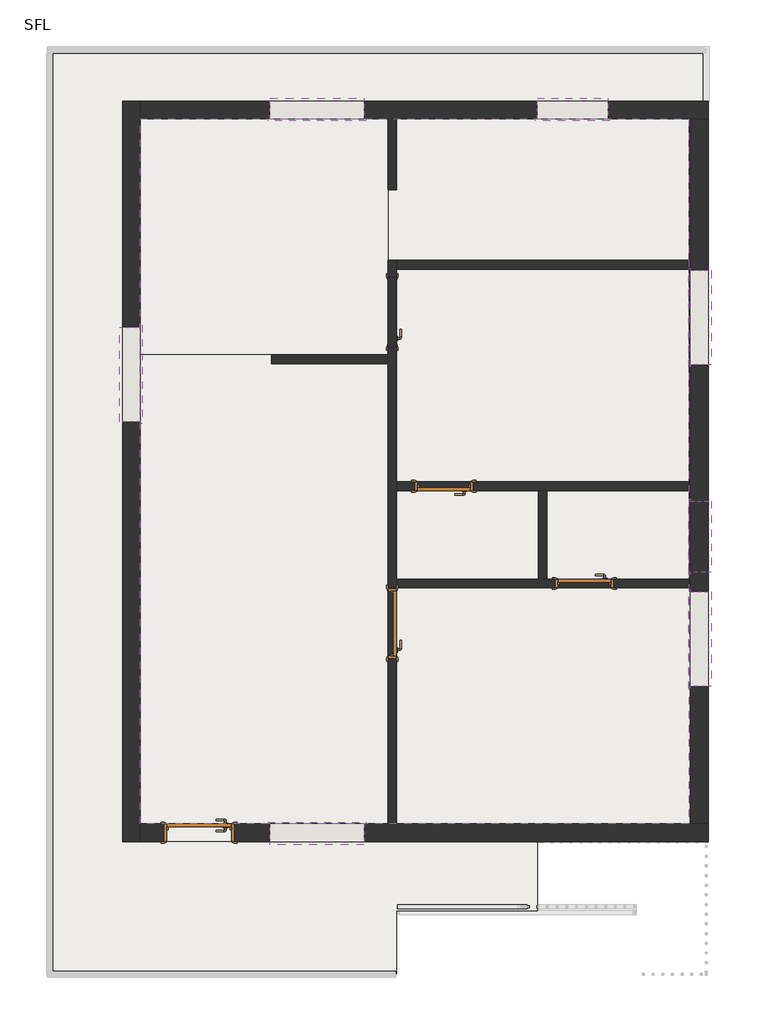
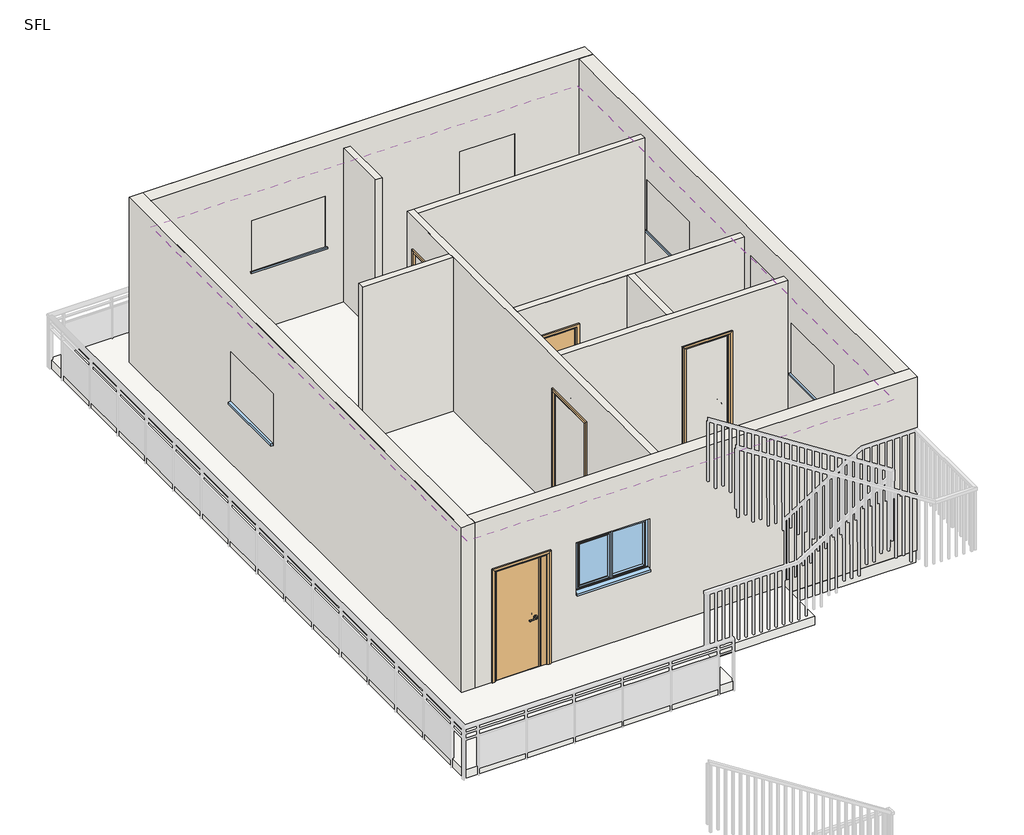
# One storey, part 1 of 4: 21 walls, 16 slabs, 7 windows, 5 doors, 1 covering.
"""IFC4 building model written with IfcOpenShell, lengths in millimetres."""

from ifc_helpers import new_model, si_unit, frame, origin, place, context, project, spatial, polyline, outline, extrude, faceted_brep, transform, mapped, element, save
from components import doors_intsgl_d1_d2de26da, doors_intsgl_d1_5aeab8eb, doors_intsgl_d2_21b53886, doors_intsgl_d2_1f5f3f16, windows_dbl_plain_w1_9e0d93ab, windows_dbl_plain_w2_c69f14ef, windows_sgl_plain_v_28d0678b

model = new_model("IFC4")

# Units and contexts
model_context = context("Model", 3, world=origin())
ifc_project = project(units=[si_unit("LENGTHUNIT", "METRE", prefix="MILLI")], contexts=[model_context])

# Site, building, storey
site = spatial("IfcSite", under=ifc_project)
building = spatial("IfcBuilding", under=site)
storey = spatial("IfcBuildingStorey", under=building, Name="SFL", Elevation=6583.68)

# Covering
placement = place(None, origin())
element("IfcCovering", 1, at=placement, inside=storey, context=model_context, shape_type="SweptSolid", body=[
    extrude(outline(polyline([(-6724.0132565, -885.5593981), (-6724.0132565, -9991.0521308), (-10495.9340108, -9991.0521308), (-13810.6009005, -9991.0521308), (-13810.6009005, -885.5593981), (-6724.0132565, -885.5593981)])), frame((0.0, 0.0, 9174.48), z_axis=(0.0, 0.0, 1.0), x_axis=(1.0, 0.0, 0.0)), (0.0, 0.0, 1.0), 57.0),
])

# Doors
doors_intsgl_d1_shape = doors_intsgl_d1_d2de26da(model_context)
element("IfcDoor", 2, ObjectType="Doors_IntSgl : D1", at=placement, inside=storey, context=model_context, shape_type="MappedRepresentation", body=[
    mapped(doors_intsgl_d1_shape, transform((-10553.0840108, -7400.866169, 6733.6416), x_axis=(0.0, 1.0, 0.0), y_axis=(-1.0, 0.0, 0.0), z_axis=(0.0, 0.0, 1.0))),
])
element("IfcDoor", 3, ObjectType="Doors_IntSgl : D1", at=placement, inside=storey, context=model_context, shape_type="MappedRepresentation", body=[
    mapped(doors_intsgl_d1_shape, transform((-10553.0840108, -3381.2262014, 6733.6416), x_axis=(0.0, 1.0, 0.0), y_axis=(-1.0, 0.0, 0.0), z_axis=(0.0, 0.0, 1.0))),
])
doors_intsgl_d1_2_shape = doors_intsgl_d1_5aeab8eb(model_context)
element("IfcDoor", 4, ObjectType="Doors_IntSgl : D1", at=placement, inside=storey, context=model_context, shape_type="MappedRepresentation", body=[
    mapped(doors_intsgl_d1_2_shape, transform((-13048.4335145, -10105.3521308, 6583.68), x_axis=(-1.0, 0.0, 0.0), y_axis=(0.0, -1.0, 0.0), z_axis=(0.0, 0.0, 1.0))),
])
doors_intsgl_d2_shape = doors_intsgl_d2_21b53886(model_context)
element("IfcDoor", 5, ObjectType="Doors_IntSgl : D2", at=placement, inside=storey, context=model_context, shape_type="MappedRepresentation", body=[
    mapped(doors_intsgl_d2_shape, transform((-9886.3340108, -5628.9784114, 6733.6416), x_axis=(-1.0, 0.0, 0.0), y_axis=(0.0, -1.0, 0.0), z_axis=(0.0, 0.0, 1.0))),
])
doors_intsgl_d2_2_shape = doors_intsgl_d2_1f5f3f16(model_context)
element("IfcDoor", 6, ObjectType="Doors_IntSgl : D2", at=placement, inside=storey, context=model_context, shape_type="MappedRepresentation", body=[
    mapped(doors_intsgl_d2_2_shape, transform((-8070.4366309, -6886.516169, 6733.6416), x_axis=(-1.0, 0.0, 0.0), y_axis=(0.0, -1.0, 0.0), z_axis=(0.0, 0.0, 1.0))),
])

# Slabs
element("IfcSlab", 7, ObjectType="BATHROOM FLOORING", at=placement, inside=storey, context=model_context, shape_type="SweptSolid", body=[
    extrude(outline(polyline([(-8667.3366309, -5686.1284114), (-8667.3366309, -6829.366169), (-10495.9340108, -6829.366169), (-10495.9340108, -5686.1284114), (-8667.3366309, -5686.1284114)])), frame((0.0, 0.0, 6583.68), z_axis=(0.0, 0.0, 1.0), x_axis=(1.0, 0.0, 0.0)), (0.0, 0.0, 1.0), 149.9616),
])
element("IfcSlab", 8, ObjectType="BATHROOM FLOORING", at=placement, inside=storey, context=model_context, shape_type="SweptSolid", body=[
    extrude(outline(polyline([(-6724.371003, -5686.0601635), (-6724.371003, -6829.366169), (-8553.0366309, -6829.366169), (-8553.0366309, -5686.0601635), (-6724.371003, -5686.0601635)])), frame((0.0, 0.0, 6583.68), z_axis=(0.0, 0.0, 1.0), x_axis=(1.0, 0.0, 0.0)), (0.0, 0.0, 1.0), 149.9616),
])
element("IfcSlab", 9, ObjectType="BATHROOM FLOORING", at=placement, inside=storey, context=model_context, shape_type="SweptSolid", body=[
    extrude(outline(polyline([(-8667.3366309, -5686.1284114), (-8667.3366309, -6829.366169), (-10495.9340108, -6829.366169), (-10495.9340108, -5686.1284114), (-8667.3366309, -5686.1284114)])), frame((0.0, 0.0, 6583.68), z_axis=(0.0, 0.0, 1.0), x_axis=(1.0, 0.0, 0.0)), (0.0, 0.0, 1.0), 149.9616),
])
element("IfcSlab", 10, ObjectType="BATHROOM FLOORING", at=placement, inside=storey, context=model_context, shape_type="SweptSolid", body=[
    extrude(outline(polyline([(-6724.371003, -5686.0601635), (-6724.371003, -6829.366169), (-8553.0366309, -6829.366169), (-8553.0366309, -5686.0601635), (-6724.371003, -5686.0601635)])), frame((0.0, 0.0, 6583.68), z_axis=(0.0, 0.0, 1.0), x_axis=(1.0, 0.0, 0.0)), (0.0, 0.0, 1.0), 149.9616),
])
element("IfcSlab", 11, ObjectType="BED ROOM FLOORING", at=placement, inside=storey, context=model_context, shape_type="SweptSolid", body=[
    extrude(outline(polyline([(-6724.371003, -2828.9136626), (-6724.371003, -5571.8284114), (-10495.9340108, -5571.8284114), (-10495.9340108, -2828.9136626), (-6724.371003, -2828.9136626)])), frame((0.0, 0.0, 6583.68), z_axis=(0.0, 0.0, 1.0), x_axis=(1.0, 0.0, 0.0)), (0.0, 0.0, 1.0), 149.9616),
])
element("IfcSlab", 12, ObjectType="BED ROOM FLOORING", at=placement, inside=storey, context=model_context, shape_type="SweptSolid", body=[
    extrude(outline(polyline([(-6698.6395131, -6943.5979211), (-6698.6395131, -9991.1886267), (-10495.9340108, -9991.1886267), (-10495.9340108, -6943.5979211), (-6698.6395131, -6943.5979211)])), frame((0.0, 0.0, 6583.68), z_axis=(0.0, 0.0, 1.0), x_axis=(1.0, 0.0, 0.0)), (0.0, 0.0, 1.0), 149.9616),
])
element("IfcSlab", 13, ObjectType="BED ROOM FLOORING", at=placement, inside=storey, context=model_context, shape_type="SweptSolid", body=[
    extrude(outline(polyline([(-6724.371003, -2828.9136626), (-6724.371003, -5571.8284114), (-10495.9340108, -5571.8284114), (-10495.9340108, -2828.9136626), (-6724.371003, -2828.9136626)])), frame((0.0, 0.0, 6583.68), z_axis=(0.0, 0.0, 1.0), x_axis=(1.0, 0.0, 0.0)), (0.0, 0.0, 1.0), 149.9616),
])
element("IfcSlab", 14, ObjectType="BED ROOM FLOORING", at=placement, inside=storey, context=model_context, shape_type="SweptSolid", body=[
    extrude(outline(polyline([(-6698.6395131, -6943.5979211), (-6698.6395131, -9991.1886267), (-10495.9340108, -9991.1886267), (-10495.9340108, -6943.5979211), (-6698.6395131, -6943.5979211)])), frame((0.0, 0.0, 6583.68), z_axis=(0.0, 0.0, 1.0), x_axis=(1.0, 0.0, 0.0)), (0.0, 0.0, 1.0), 149.9616),
])
element("IfcSlab", 15, ObjectType="DINING FLOORING", at=placement, inside=storey, context=model_context, shape_type="SweptSolid", body=[
    extrude(outline(polyline([(-10610.2340108, -885.9480347), (-10610.2340108, -3933.5387403), (-13810.6009005, -3933.5387403), (-13810.6009005, -885.9480347), (-10610.2340108, -885.9480347)])), frame((0.0, 0.0, 6583.68), z_axis=(0.0, 0.0, 1.0), x_axis=(1.0, 0.0, 0.0)), (0.0, 0.0, 1.0), 149.9616),
])
element("IfcSlab", 16, ObjectType="DINING FLOORING", at=placement, inside=storey, context=model_context, shape_type="SweptSolid", body=[
    extrude(outline(polyline([(-10610.2340108, -885.9480347), (-10610.2340108, -3933.5387403), (-13810.6009005, -3933.5387403), (-13810.6009005, -885.9480347), (-10610.2340108, -885.9480347)])), frame((0.0, 0.0, 6583.68), z_axis=(0.0, 0.0, 1.0), x_axis=(1.0, 0.0, 0.0)), (0.0, 0.0, 1.0), 149.9616),
])
element("IfcSlab", 17, ObjectType="HALL FLOORING", at=placement, inside=storey, context=model_context, shape_type="SweptSolid", body=[
    extrude(outline(polyline([(-10610.2340108, -3933.5387403), (-10610.2340108, -9991.0521308), (-13810.6009005, -9991.0521308), (-13810.6009005, -3933.5387403), (-10610.2340108, -3933.5387403)])), frame((0.0, 0.0, 6583.68), z_axis=(0.0, 0.0, 1.0), x_axis=(1.0, 0.0, 0.0)), (0.0, 0.0, 1.0), 149.9616),
])
element("IfcSlab", 18, ObjectType="HALL FLOORING", at=placement, inside=storey, context=model_context, shape_type="SweptSolid", body=[
    extrude(outline(polyline([(-10610.2340108, -3933.5387403), (-10610.2340108, -9991.0521308), (-13810.6009005, -9991.0521308), (-13810.6009005, -3933.5387403), (-10610.2340108, -3933.5387403)])), frame((0.0, 0.0, 6583.68), z_axis=(0.0, 0.0, 1.0), x_axis=(1.0, 0.0, 0.0)), (0.0, 0.0, 1.0), 149.9616),
])
element("IfcSlab", 19, ObjectType="KITCHEN FLOOR", at=placement, inside=storey, context=model_context, shape_type="SweptSolid", body=[
    extrude(outline(polyline([(-6724.371003, -885.9480347), (-6724.371003, -2714.6136626), (-10495.9340108, -2714.6136626), (-10610.2340108, -2714.6136626), (-10610.2340108, -1800.3480347), (-10495.9340108, -1800.3480347), (-10495.9340108, -885.9480347), (-6724.371003, -885.9480347)])), frame((0.0, 0.0, 6583.68), z_axis=(0.0, 0.0, 1.0), x_axis=(1.0, 0.0, 0.0)), (0.0, 0.0, 1.0), 149.9616),
])
element("IfcSlab", 20, ObjectType="KITCHEN FLOOR", at=placement, inside=storey, context=model_context, shape_type="SweptSolid", body=[
    extrude(outline(polyline([(-6724.371003, -885.9480347), (-6724.371003, -2714.6136626), (-10495.9340108, -2714.6136626), (-10610.2340108, -2714.6136626), (-10610.2340108, -1800.3480347), (-10495.9340108, -1800.3480347), (-10495.9340108, -885.9480347), (-6724.371003, -885.9480347)])), frame((0.0, 0.0, 6583.68), z_axis=(0.0, 0.0, 1.0), x_axis=(1.0, 0.0, 0.0)), (0.0, 0.0, 1.0), 149.9616),
])
element("IfcSlab", 21, ObjectType="OUTER FLOORING", at=placement, inside=storey, context=model_context, shape_type="SweptSolid", body=[
    extrude(outline(polyline([(-6495.4132565, 3.4571089), (-6495.4132565, -656.9593981), (-14039.0335145, -656.9593981), (-14039.0335145, -10219.6521308), (-8680.149573, -10219.6521308), (-8680.149573, -11109.5255223), (-10495.9340108, -11109.5255223), (-10495.9340108, -11928.1928911), (-14979.3420435, -11928.1928911), (-14979.3420435, 3.4571089), (-6495.4132565, 3.4571089)])), frame((0.0, 0.0, 6583.68), z_axis=(0.0, 0.0, 1.0), x_axis=(1.0, 0.0, 0.0)), (0.0, 0.0, 1.0), 149.9616),
])
element("IfcSlab", 22, ObjectType="RCC SLAB", at=placement, inside=storey, context=model_context, shape_type="SweptSolid", body=[
    extrude(outline(polyline([(-6495.4132565, -656.9593981), (-6495.4132565, -10219.6521308), (-14039.0335145, -10219.6521308), (-14039.0335145, -656.9593981), (-6495.4132565, -656.9593981)])), frame((0.0, 0.0, 6383.7312), z_axis=(0.0, 0.0, 1.0), x_axis=(1.0, 0.0, 0.0)), (0.0, 0.0, 1.0), 199.9488),
])

# Walls
element("IfcWall", 23, ObjectType="EXT WALL", at=placement, inside=storey, context=model_context, shape_type="Brep", body=[
    faceted_brep([(-14039.0335145, -656.9593981, 6583.68), (-14039.0335145, -10219.6521308, 6583.68), (-14039.0335145, -10219.6521308, 9631.68), (-14039.0335145, -656.9593981, 9631.68), (-14039.0335145, -4797.1593981, 8693.68), (-14039.0335145, -4797.1593981, 7783.68), (-14039.0335145, -3577.9593981, 7783.68), (-14039.0335145, -3577.9593981, 8693.68), (-13810.4335145, -656.9593981, 6583.68), (-13810.4335145, -656.9593981, 9631.68), (-13810.4335145, -885.5593981, 9631.68), (-13810.4335145, -9991.0521308, 9631.68), (-13810.4335145, -10219.6521308, 9631.68), (-13810.4335145, -10219.6521308, 6583.68), (-13810.4335145, -9991.0521308, 6583.68), (-13810.4335145, -885.5593981, 6583.68), (-13810.4335145, -4797.1593981, 8693.68), (-13810.4335145, -3577.9593981, 8693.68), (-13810.4335145, -3577.9593981, 7783.68), (-13810.4335145, -4797.1593981, 7783.68)], [[[0, 1, 2, 3], [4, 5, 6, 7]], [[8, 9, 10, 11, 12, 13, 14, 15], [16, 17, 18, 19]], [[1, 0, 8, 15, 14, 13]], [[3, 2, 12, 11, 10, 9]], [[2, 1, 13, 12]], [[0, 3, 9, 8]], [[5, 4, 16, 19]], [[6, 5, 19, 18]], [[7, 6, 18, 17]], [[4, 7, 17, 16]]]),
])
element("IfcWall", 24, ObjectType="EXT WALL", at=placement, inside=storey, context=model_context, shape_type="Brep", body=[
    faceted_brep([(-13810.4335145, -9991.0521308, 9631.68), (-6698.971003, -9991.0521308, 9631.68), (-6470.371003, -9991.0521308, 9631.68), (-6470.371003, -9991.0521308, 6583.68), (-6698.971003, -9991.0521308, 6583.68), (-10495.9340108, -9991.0521308, 6583.68), (-10610.2340108, -9991.0521308, 6583.68), (-12591.2335145, -9991.0521308, 6583.68), (-12591.2335145, -9991.0521308, 8693.68), (-13505.6335145, -9991.0521308, 8693.68), (-13505.6335145, -9991.0521308, 6583.68), (-13810.4335145, -9991.0521308, 6583.68), (-10915.0340108, -9991.0521308, 7783.68), (-10915.0340108, -9991.0521308, 8693.68), (-12134.2340108, -9991.0521308, 8693.68), (-12134.2340108, -9991.0521308, 7783.68), (-6470.371003, -10219.6521308, 9631.68), (-13810.4335145, -10219.6521308, 9631.68), (-13810.4335145, -10219.6521308, 6583.68), (-13505.6335145, -10219.6521308, 6583.68), (-13505.6335145, -10219.6521308, 8693.68), (-12591.2335145, -10219.6521308, 8693.68), (-12591.2335145, -10219.6521308, 6583.68), (-6470.371003, -10219.6521308, 6583.68), (-10915.0340108, -10219.6521308, 8693.68), (-10915.0340108, -10219.6521308, 7783.68), (-12134.2340108, -10219.6521308, 7783.68), (-12134.2340108, -10219.6521308, 8693.68)], [[[0, 1, 2, 3, 4, 5, 6, 7, 8, 9, 10, 11], [12, 13, 14, 15]], [[16, 17, 18, 19, 20, 21, 22, 23], [24, 25, 26, 27]], [[18, 11, 10, 19]], [[3, 23, 22, 7, 6, 5, 4]], [[2, 1, 0, 17, 16]], [[0, 11, 18, 17]], [[3, 2, 16, 23]], [[25, 24, 13, 12]], [[26, 25, 12, 15]], [[27, 26, 15, 14]], [[24, 27, 14, 13]], [[9, 20, 19, 10]], [[20, 9, 8, 21]], [[21, 8, 7, 22]]]),
])
element("IfcWall", 25, ObjectType="EXT WALL", at=placement, inside=storey, context=model_context, shape_type="Brep", body=[
    faceted_brep([(-13810.4335145, -885.5593981, 6583.68), (-6698.971003, -885.5593981, 6583.68), (-6470.371003, -885.5593981, 6583.68), (-6470.371003, -885.5593981, 9631.68), (-6698.971003, -885.5593981, 9631.68), (-13810.4335145, -885.5593981, 9631.68), (-8679.8132565, -885.5593981, 8693.68), (-7765.4132565, -885.5593981, 8693.68), (-7765.4132565, -885.5593981, 7783.68), (-8679.8132565, -885.5593981, 7783.68), (-12134.0335145, -885.5593981, 8693.68), (-10914.8335145, -885.5593981, 8693.68), (-10914.8335145, -885.5593981, 7783.68), (-12134.0335145, -885.5593981, 7783.68), (-13810.4335145, -656.9593981, 6583.68), (-13810.4335145, -656.9593981, 9631.68), (-6470.371003, -656.9593981, 9631.68), (-6470.371003, -656.9593981, 6583.68), (-8679.8132565, -656.9593981, 8693.68), (-8679.8132565, -656.9593981, 7783.68), (-7765.4132565, -656.9593981, 7783.68), (-7765.4132565, -656.9593981, 8693.68), (-12134.0335145, -656.9593981, 8693.68), (-12134.0335145, -656.9593981, 7783.68), (-10914.8335145, -656.9593981, 7783.68), (-10914.8335145, -656.9593981, 8693.68)], [[[0, 1, 2, 3, 4, 5], [6, 7, 8, 9], [10, 11, 12, 13]], [[14, 15, 16, 17], [18, 19, 20, 21], [22, 23, 24, 25]], [[2, 1, 0, 14, 17]], [[5, 4, 3, 16, 15]], [[0, 5, 15, 14]], [[3, 2, 17, 16]], [[19, 18, 6, 9]], [[20, 19, 9, 8]], [[21, 20, 8, 7]], [[18, 21, 7, 6]], [[23, 22, 10, 13]], [[24, 23, 13, 12]], [[25, 24, 12, 11]], [[22, 25, 11, 10]]]),
])
element("IfcWall", 26, ObjectType="EXT WALL", at=placement, inside=storey, context=model_context, shape_type="SweptSolid", body=[
    extrude(outline(polyline([(-885.5593981, 6583.68), (-9991.0521308, 6583.68), (-9991.0521308, 9631.68), (-885.5593981, 9631.68), (-885.5593981, 6583.68)]), holes=[polyline([(-5825.4521308, 9170.08), (-6739.8521308, 9170.08), (-6739.8521308, 8260.08), (-5825.4521308, 8260.08), (-5825.4521308, 9170.08)]), polyline([(-2841.3593981, 8693.68), (-4060.5593981, 8693.68), (-4060.5593981, 7783.68), (-2841.3593981, 7783.68), (-2841.3593981, 8693.68)]), polyline([(-6993.8521308, 8693.68), (-8213.0521308, 8693.68), (-8213.0521308, 7783.68), (-6993.8521308, 7783.68), (-6993.8521308, 8693.68)])]), frame((-6698.971003, 0.0, 0.0), z_axis=(1.0, 0.0, 0.0), x_axis=(0.0, 1.0, 0.0)), (0.0, 0.0, 1.0), 228.6),
])
element("IfcWall", 27, ObjectType="EXT WALL", at=placement, inside=storey, context=model_context, shape_type="SweptSolid", body=[
    extrude(outline(polyline([(-14039.0335145, -9991.0521308), (-14039.0335145, -885.5593981), (-13810.4335145, -885.5593981), (-13810.4335145, -9991.0521308), (-14039.0335145, -9991.0521308)])), frame((0.0, 0.0, 6583.68), z_axis=(0.0, 0.0, 1.0), x_axis=(1.0, 0.0, 0.0)), (0.0, 0.0, 1.0), 3048.0),
])
element("IfcWall", 28, ObjectType="EXT WALL", at=placement, inside=storey, context=model_context, shape_type="SweptSolid", body=[
    extrude(outline(polyline([(-6698.971003, -885.5593981), (-13810.4335145, -885.5593981), (-13810.4335145, -656.9593981), (-6698.971003, -656.9593981), (-6698.971003, -885.5593981)])), frame((0.0, 0.0, 6583.68), z_axis=(0.0, 0.0, 1.0), x_axis=(1.0, 0.0, 0.0)), (0.0, 0.0, 1.0), 3048.0),
])
element("IfcWall", 29, ObjectType="EXT WALL", at=placement, inside=storey, context=model_context, shape_type="SweptSolid", body=[
    extrude(outline(polyline([(-6698.971003, -9991.0521308), (-6698.971003, -885.5593981), (-6470.371003, -885.5593981), (-6470.371003, -9991.0521308), (-6698.971003, -9991.0521308)])), frame((0.0, 0.0, 6583.68), z_axis=(0.0, 0.0, 1.0), x_axis=(1.0, 0.0, 0.0)), (0.0, 0.0, 1.0), 3048.0),
])
element("IfcWall", 30, ObjectType="INT WALL", at=placement, inside=storey, context=model_context, shape_type="SweptSolid", body=[
    extrude(outline(polyline([(-10610.2340108, -1800.3480347), (-10610.2340108, -885.9480347), (-10495.9340108, -885.9480347), (-10495.9340108, -1800.3480347), (-10610.2340108, -1800.3480347)])), frame((0.0, 0.0, 6583.68), z_axis=(0.0, 0.0, 1.0), x_axis=(1.0, 0.0, 0.0)), (0.0, 0.0, 1.0), 2848.0512),
])
element("IfcWall", 31, ObjectType="INT WALL", at=placement, inside=storey, context=model_context, shape_type="SweptSolid", body=[
    extrude(outline(polyline([(-10495.9340108, -2714.6136626), (-6724.371003, -2714.6136626), (-6724.371003, -2828.9136626), (-10495.9340108, -2828.9136626), (-10495.9340108, -2714.6136626)])), frame((0.0, 0.0, 6583.68), z_axis=(0.0, 0.0, 1.0), x_axis=(1.0, 0.0, 0.0)), (0.0, 0.0, 1.0), 2848.0512),
])
element("IfcWall", 32, ObjectType="INT WALL", at=placement, inside=storey, context=model_context, shape_type="Brep", body=[
    faceted_brep([(-10495.9340108, -5686.1284114, 6583.68), (-8667.3366309, -5686.1284114, 6583.68), (-8553.0366309, -5686.1284114, 6583.68), (-6724.371003, -5686.1284114, 6583.68), (-6724.371003, -5686.1284114, 9431.7312), (-10495.9340108, -5686.1284114, 9431.7312), (-10267.3340108, -5686.1284114, 6733.6416), (-10267.3340108, -5686.1284114, 8843.6416), (-9505.3340108, -5686.1284114, 8843.6416), (-9505.3340108, -5686.1284114, 6733.6416), (-6724.371003, -5571.8284114, 6583.68), (-10495.9340108, -5571.8284114, 6583.68), (-10495.9340108, -5571.8284114, 9431.7312), (-6724.371003, -5571.8284114, 9431.7312), (-10267.3340108, -5571.8284114, 8843.6416), (-10267.3340108, -5571.8284114, 6733.6416), (-9505.3340108, -5571.8284114, 6733.6416), (-9505.3340108, -5571.8284114, 8843.6416)], [[[0, 1, 2, 3, 4, 5], [6, 7, 8, 9]], [[10, 11, 12, 13], [14, 15, 16, 17]], [[3, 2, 1, 0, 11, 10]], [[3, 10, 13, 4]], [[11, 0, 5, 12]], [[6, 15, 14, 7]], [[7, 14, 17, 8]], [[16, 9, 8, 17]], [[15, 6, 9, 16]], [[5, 4, 13, 12]]]),
])
element("IfcWall", 33, ObjectType="INT WALL", at=placement, inside=storey, context=model_context, shape_type="Brep", body=[
    faceted_brep([(-10495.9340108, -6943.666169, 6587.0136234), (-6724.371003, -6943.666169, 6587.0136234), (-6724.371003, -6943.666169, 9431.7312), (-10495.9340108, -6943.666169, 9431.7312), (-10495.9340108, -6943.666169, 8843.6416), (-10495.9340108, -6943.666169, 6733.6416), (-8451.4366309, -6943.666169, 6733.6416), (-8451.4366309, -6943.666169, 8843.6416), (-7689.4366309, -6943.666169, 8843.6416), (-7689.4366309, -6943.666169, 6733.6416), (-6724.371003, -6829.366169, 6587.0136234), (-10495.9340108, -6829.366169, 6587.0136234), (-10495.9340108, -6829.366169, 9431.7312), (-8667.3366309, -6829.366169, 9431.7312), (-8553.0366309, -6829.366169, 9431.7312), (-6724.371003, -6829.366169, 9431.7312), (-8451.4366309, -6829.366169, 8843.6416), (-8451.4366309, -6829.366169, 6733.6416), (-7689.4366309, -6829.366169, 6733.6416), (-7689.4366309, -6829.366169, 8843.6416)], [[[0, 1, 2, 3, 4, 5], [6, 7, 8, 9]], [[10, 11, 12, 13, 14, 15], [16, 17, 18, 19]], [[1, 0, 11, 10]], [[1, 10, 15, 2]], [[11, 0, 5, 4, 3, 12]], [[6, 17, 16, 7]], [[7, 16, 19, 8]], [[18, 9, 8, 19]], [[17, 6, 9, 18]], [[3, 2, 15, 14, 13, 12]]]),
])
element("IfcWall", 34, ObjectType="INT WALL", at=placement, inside=storey, context=model_context, shape_type="SweptSolid", body=[
    extrude(outline(polyline([(-8667.3366309, -6829.366169), (-8667.3366309, -5686.1284114), (-8553.0366309, -5686.1284114), (-8553.0366309, -6829.366169), (-8667.3366309, -6829.366169)])), frame((0.0, 0.0, 6583.68), z_axis=(0.0, 0.0, 1.0), x_axis=(1.0, 0.0, 0.0)), (0.0, 0.0, 1.0), 2848.0512),
])
element("IfcWall", 35, ObjectType="INT WALL", at=placement, inside=storey, context=model_context, shape_type="SweptSolid", body=[
    extrude(outline(polyline([(-10610.2340108, -4047.8387403), (-12112.7859221, -4047.8387403), (-12112.7859221, -3933.5387403), (-10610.2340108, -3933.5387403), (-10610.2340108, -4047.8387403)])), frame((0.0, 0.0, 6583.68), z_axis=(0.0, 0.0, 1.0), x_axis=(1.0, 0.0, 0.0)), (0.0, 0.0, 1.0), 2848.0512),
])
element("IfcWall", 36, ObjectType="INT WALL", at=placement, inside=storey, context=model_context, shape_type="Brep", body=[
    faceted_brep([(-10610.2340108, -2714.6136626, 6583.68), (-10610.2340108, -3933.5387403, 6583.68), (-10610.2340108, -4047.8387403, 6583.68), (-10610.2340108, -9991.0521308, 6583.68), (-10610.2340108, -9991.0521308, 9431.7312), (-10610.2340108, -4047.8387403, 9431.7312), (-10610.2340108, -3933.5387403, 9431.7312), (-10610.2340108, -2714.6136626, 9431.7312), (-10610.2340108, -7858.066169, 6733.6416), (-10610.2340108, -6943.666169, 6733.6416), (-10610.2340108, -6943.666169, 8843.6416), (-10610.2340108, -7858.066169, 8843.6416), (-10610.2340108, -3838.4262014, 6733.6416), (-10610.2340108, -2924.0262014, 6733.6416), (-10610.2340108, -2924.0262014, 8843.6416), (-10610.2340108, -3838.4262014, 8843.6416), (-10495.9340108, -9991.0521308, 6583.68), (-10495.9340108, -5686.1284114, 6583.68), (-10495.9340108, -5571.8284114, 6583.68), (-10495.9340108, -2828.9136626, 6583.68), (-10495.9340108, -2714.6136626, 6583.68), (-10495.9340108, -2714.6136626, 9431.7312), (-10495.9340108, -2828.9136626, 9431.7312), (-10495.9340108, -5571.8284114, 9431.7312), (-10495.9340108, -5686.1284114, 9431.7312), (-10495.9340108, -6829.366169, 9431.7312), (-10495.9340108, -6943.666169, 9431.7312), (-10495.9340108, -9991.0521308, 9431.7312), (-10495.9340108, -6943.666169, 6733.6416), (-10495.9340108, -7858.066169, 6733.6416), (-10495.9340108, -7858.066169, 8843.6416), (-10495.9340108, -6943.666169, 8843.6416), (-10495.9340108, -2924.0262014, 6733.6416), (-10495.9340108, -3838.4262014, 6733.6416), (-10495.9340108, -3838.4262014, 8843.6416), (-10495.9340108, -2924.0262014, 8843.6416)], [[[0, 1, 2, 3, 4, 5, 6, 7], [8, 9, 10, 11], [12, 13, 14, 15]], [[16, 17, 18, 19, 20, 21, 22, 23, 24, 25, 26, 27], [28, 29, 30, 31], [32, 33, 34, 35]], [[3, 2, 1, 0, 20, 19, 18, 17, 16]], [[3, 16, 27, 4]], [[9, 8, 29, 28]], [[8, 11, 30, 29]], [[11, 10, 31, 30]], [[10, 9, 28, 31]], [[13, 12, 33, 32]], [[12, 15, 34, 33]], [[15, 14, 35, 34]], [[14, 13, 32, 35]], [[20, 0, 7, 21]], [[7, 6, 5, 4, 27, 26, 25, 24, 23, 22, 21]]]),
])
element("IfcWall", 37, ObjectType="INT WALL", at=placement, inside=storey, context=model_context, shape_type="SweptSolid", body=[
    extrude(outline(polyline([(-10610.2340108, -1800.3480347), (-10610.2340108, -885.9480347), (-10495.9340108, -885.9480347), (-10495.9340108, -1800.3480347), (-10610.2340108, -1800.3480347)])), frame((0.0, 0.0, 6583.68), z_axis=(0.0, 0.0, 1.0), x_axis=(1.0, 0.0, 0.0)), (0.0, 0.0, 1.0), 2848.0512),
])
element("IfcWall", 38, ObjectType="INT WALL", at=placement, inside=storey, context=model_context, shape_type="SweptSolid", body=[
    extrude(outline(polyline([(-10495.9340108, -2714.6136626), (-6724.371003, -2714.6136626), (-6724.371003, -2828.9136626), (-10495.9340108, -2828.9136626), (-10495.9340108, -2714.6136626)])), frame((0.0, 0.0, 6583.68), z_axis=(0.0, 0.0, 1.0), x_axis=(1.0, 0.0, 0.0)), (0.0, 0.0, 1.0), 2848.0512),
])
element("IfcWall", 39, ObjectType="INT WALL", at=placement, inside=storey, context=model_context, shape_type="Brep", body=[
    faceted_brep([(-10495.9340108, -5686.1284114, 6583.68), (-8667.3366309, -5686.1284114, 6583.68), (-8553.0366309, -5686.1284114, 6583.68), (-6724.371003, -5686.1284114, 6583.68), (-6724.371003, -5686.1284114, 9431.7312), (-8553.0366309, -5686.1284114, 9431.7312), (-8667.3366309, -5686.1284114, 9431.7312), (-10495.9340108, -5686.1284114, 9431.7312), (-6724.371003, -5571.8284114, 6583.68), (-10495.9340108, -5571.8284114, 6583.68), (-10495.9340108, -5571.8284114, 9431.7312), (-6724.371003, -5571.8284114, 9431.7312)], [[[0, 1, 2, 3, 4, 5, 6, 7]], [[8, 9, 10, 11]], [[3, 2, 1, 0, 9, 8]], [[3, 8, 11, 4]], [[9, 0, 7, 10]], [[7, 6, 5, 4, 11, 10]]]),
])
element("IfcWall", 40, ObjectType="INT WALL", at=placement, inside=storey, context=model_context, shape_type="Brep", body=[
    faceted_brep([(-10495.9340108, -6943.666169, 6587.0136234), (-6724.371003, -6943.666169, 6587.0136234), (-6724.371003, -6943.666169, 9431.7312), (-10495.9340108, -6943.666169, 9431.7312), (-10495.9340108, -6943.666169, 8843.6416), (-10495.9340108, -6943.666169, 6733.6416), (-6724.371003, -6829.366169, 6587.0136234), (-10495.9340108, -6829.366169, 6587.0136234), (-10495.9340108, -6829.366169, 9431.7312), (-8667.3366309, -6829.366169, 9431.7312), (-8553.0366309, -6829.366169, 9431.7312), (-6724.371003, -6829.366169, 9431.7312)], [[[0, 1, 2, 3, 4, 5]], [[6, 7, 8, 9, 10, 11]], [[1, 0, 7, 6]], [[1, 6, 11, 2]], [[7, 0, 5, 4, 3, 8]], [[3, 2, 11, 10, 9, 8]]]),
])
element("IfcWall", 41, ObjectType="INT WALL", at=placement, inside=storey, context=model_context, shape_type="SweptSolid", body=[
    extrude(outline(polyline([(-8667.3366309, -6829.366169), (-8667.3366309, -5686.1284114), (-8553.0366309, -5686.1284114), (-8553.0366309, -6829.366169), (-8667.3366309, -6829.366169)])), frame((0.0, 0.0, 6583.68), z_axis=(0.0, 0.0, 1.0), x_axis=(1.0, 0.0, 0.0)), (0.0, 0.0, 1.0), 2848.0512),
])
element("IfcWall", 42, ObjectType="INT WALL", at=placement, inside=storey, context=model_context, shape_type="SweptSolid", body=[
    extrude(outline(polyline([(-10610.2340108, -4047.8387403), (-12112.7859221, -4047.8387403), (-12112.7859221, -3933.5387403), (-10610.2340108, -3933.5387403), (-10610.2340108, -4047.8387403)])), frame((0.0, 0.0, 6583.68), z_axis=(0.0, 0.0, 1.0), x_axis=(1.0, 0.0, 0.0)), (0.0, 0.0, 1.0), 2848.0512),
])
element("IfcWall", 43, ObjectType="INT WALL", at=placement, inside=storey, context=model_context, shape_type="Brep", body=[
    faceted_brep([(-10610.2340108, -2828.9136626, 6583.68), (-10610.2340108, -3933.5387403, 6583.68), (-10610.2340108, -4047.8387403, 6583.68), (-10610.2340108, -9991.0521308, 6583.68), (-10610.2340108, -9991.0521308, 9431.7312), (-10610.2340108, -4047.8387403, 9431.7312), (-10610.2340108, -3933.5387403, 9431.7312), (-10610.2340108, -2828.9136626, 9431.7312), (-10495.9340108, -9991.0521308, 6583.68), (-10495.9340108, -5686.1284114, 6583.68), (-10495.9340108, -5571.8284114, 6583.68), (-10495.9340108, -2828.9136626, 6583.68), (-10495.9340108, -2828.9136626, 9431.7312), (-10495.9340108, -5571.8284114, 9431.7312), (-10495.9340108, -5686.1284114, 9431.7312), (-10495.9340108, -6829.366169, 9431.7312), (-10495.9340108, -6943.666169, 9431.7312), (-10495.9340108, -9991.0521308, 9431.7312)], [[[0, 1, 2, 3, 4, 5, 6, 7]], [[8, 9, 10, 11, 12, 13, 14, 15, 16, 17]], [[3, 2, 1, 0, 11, 10, 9, 8]], [[3, 8, 17, 4]], [[11, 0, 7, 12]], [[7, 6, 5, 4, 17, 16, 15, 14, 13, 12]]]),
])

# Windows
windows_dbl_plain_w1_shape = windows_dbl_plain_w1_9e0d93ab(model_context)
element("IfcWindow", 44, ObjectType="Windows_Dbl_Plain : W1", at=placement, inside=storey, context=model_context, shape_type="MappedRepresentation", body=[
    mapped(windows_dbl_plain_w1_shape, transform((-6593.1275708, -7888.4521308, 6583.68), x_axis=(0.0, -1.0, 0.0), y_axis=(1.0, 0.0, 0.0), z_axis=(0.0, 0.0, 1.0))),
])
element("IfcWindow", 45, ObjectType="Windows_Dbl_Plain : W1", at=placement, inside=storey, context=model_context, shape_type="MappedRepresentation", body=[
    mapped(windows_dbl_plain_w1_shape, transform((-6593.1275708, -3735.9593981, 6583.68), x_axis=(0.0, -1.0, 0.0), y_axis=(1.0, 0.0, 0.0), z_axis=(0.0, 0.0, 1.0))),
])
element("IfcWindow", 46, ObjectType="Windows_Dbl_Plain : W1", at=placement, inside=storey, context=model_context, shape_type="MappedRepresentation", body=[
    mapped(windows_dbl_plain_w1_shape, transform((-11239.4335145, -779.7159659, 6583.68), x_axis=(1.0, 0.0, 0.0), y_axis=(0.0, 1.0, 0.0), z_axis=(0.0, 0.0, 1.0))),
])
element("IfcWindow", 47, ObjectType="Windows_Dbl_Plain : W1", at=placement, inside=storey, context=model_context, shape_type="MappedRepresentation", body=[
    mapped(windows_dbl_plain_w1_shape, transform((-13916.2769467, -3902.5593981, 6583.68), x_axis=(0.0, 1.0, 0.0), y_axis=(-1.0, 0.0, 0.0), z_axis=(0.0, 0.0, 1.0))),
])
element("IfcWindow", 48, ObjectType="Windows_Dbl_Plain : W1", at=placement, inside=storey, context=model_context, shape_type="MappedRepresentation", body=[
    mapped(windows_dbl_plain_w1_shape, transform((-11809.6340108, -10096.895563, 6583.68), x_axis=(-1.0, 0.0, 0.0), y_axis=(0.0, -1.0, 0.0), z_axis=(0.0, 0.0, 1.0))),
])
windows_dbl_plain_w2_shape = windows_dbl_plain_w2_c69f14ef(model_context)
element("IfcWindow", 49, ObjectType="Windows_Dbl_Plain : W2", at=placement, inside=storey, context=model_context, shape_type="MappedRepresentation", body=[
    mapped(windows_dbl_plain_w2_shape, transform((-7937.6132565, -779.7159659, 6583.68), x_axis=(1.0, 0.0, 0.0), y_axis=(0.0, 1.0, 0.0), z_axis=(0.0, 0.0, 1.0))),
])
windows_sgl_plain_v_shape = windows_sgl_plain_v_28d0678b(model_context)
element("IfcWindow", 50, ObjectType="Windows_Sgl_Plain : V", at=placement, inside=storey, context=model_context, shape_type="MappedRepresentation", body=[
    mapped(windows_sgl_plain_v_shape, transform((-6593.1275708, -6282.6521308, 7060.08), x_axis=(0.0, -1.0, 0.0), y_axis=(1.0, 0.0, 0.0), z_axis=(0.0, 0.0, 1.0))),
])

save(model, "model.ifc")

# Revit data of these elements
# Type
#   Keynote = "K40"
#   built-in parameter 1002203 = 1 (stored number, unit not read)
#   built-in parameter 1002202 = 1 (stored number, unit not read)
#   Layers, outside or top first: 0.147638 ft "Metal Stud Layer" (function 1); 0.03937 ft "Gypsum Wall Board" (function 1)
# Type "Doors_IntSgl : D1"
#   Type Mark = "46"
#   Type Comments = "Internal Single"
#   Operation = "SingleSwingRight"
#   Manufacturer = "Revit"
#   Keynote = "L20"
#   Description = "Internal Single Door"
#   Analytic Construction = "Metal"
#   UnderCut = 0.026247 ft
#   Tolerance = 0.006562 ft
#   Thickness = 0.124672 ft
#   Thermal Resistance (R) = 0.270117 (m²·K)/W
#   Structural Tolerance = 0.026247 ft
#   StopDepth = 0.104987 ft
#   Stop Thickness = 0.062336 ft
#   Rough Width = 3.0 ft
#   Rough Height = 6.922572 ft
#   Height to Top Lock Rail = 3.28084 ft
#   Heat Transfer Coefficient (U) = 3.7021 W/(m²·K)
#   Handle Z Distance = 2.952756 ft
#   Handle X Distance = 0.246063 ft
#   Frame Thickness = 0.104987 ft
#   Door Panel Width = 2.724409 ft
#   Door Panel Thickness = 0.124672 ft
#   Door Panel Offset = 0.0 ft
#   Height = 6.922572 ft
#   Width = 3.0 ft
#   Door Panel Height = 6.75853 ft
#   Architrave Setback = 0.016404 ft
#   Vis - Ironmongery = yes
#   Material Ironmongery = Door - Handle
#   Material Frame = Door - Frame/Mullion (1)
#   Material Door = Door - Panel
#   Material Architrave = Door - Architrave
#   Visual Light Transmittance = 0
#   Solar Heat Gain Coefficient = 0
#   Function = (empty or 0)
#   Wall Closure = (empty or 0)
# Type "Doors_IntSgl : D2"
#   Type Mark = "47"
#   Type Comments = "Internal Single"
#   Operation = "SingleSwingRight"
#   Manufacturer = "Revit"
#   Keynote = "L20"
#   Description = "Internal Single Door"
#   Analytic Construction = "Metal"
#   UnderCut = 0.026247 ft
#   Tolerance = 0.006562 ft
#   Thickness = 0.124672 ft
#   Thermal Resistance (R) = 0.270117 (m²·K)/W
#   Structural Tolerance = 0.026247 ft
#   StopDepth = 0.104987 ft
#   Stop Thickness = 0.062336 ft
#   Rough Width = 2.5 ft
#   Rough Height = 6.922572 ft
#   Height to Top Lock Rail = 3.28084 ft
#   Heat Transfer Coefficient (U) = 3.7021 W/(m²·K)
#   Handle Z Distance = 2.952756 ft
#   Handle X Distance = 0.246063 ft
#   Frame Thickness = 0.104987 ft
#   Door Panel Width = 2.224409 ft
#   Door Panel Thickness = 0.124672 ft
#   Door Panel Offset = 0.0 ft
#   Height = 6.922572 ft
#   Width = 2.5 ft
#   Door Panel Height = 6.75853 ft
#   Architrave Setback = 0.016404 ft
#   Vis - Ironmongery = yes
#   Material Ironmongery = Door - Handle
#   Material Frame = Door - Frame/Mullion (1)
#   Material Door = Door - Panel
#   Material Architrave = Door - Architrave
#   Visual Light Transmittance = 0
#   Solar Heat Gain Coefficient = 0
#   Function = (empty or 0)
#   Wall Closure = (empty or 0)
# Type "BATHROOM FLOORING"
#   Function = 0
#   Layers, outside or top first: 0.072 ft "BATHROOM FLOOR" (function 5); 0.42 ft "Structure, Timber Joist/Rafter Layer" (function 1)
# Type "BED ROOM FLOORING"
#   Function = 0
#   Layers, outside or top first: 0.072 ft "BEDROOM FLOOR" (function 5); 0.42 ft "Structure, Timber Joist/Rafter Layer" (function 1)
# Type "DINING FLOORING"
#   Function = 0
#   Layers, outside or top first: 0.072 ft "KITCHEN FLOOR" (function 5); 0.42 ft "Structure, Timber Joist/Rafter Layer" (function 1)
# Type "HALL FLOORING"
#   Function = 0
#   Layers, outside or top first: 0.072 ft "HALL FLOOR" (function 5); 0.42 ft "Structure, Timber Joist/Rafter Layer" (function 1)
# Type "KITCHEN FLOOR"
#   Function = 0
#   Layers, outside or top first: 0.072 ft "KITCHEN FLOOR" (function 5); 0.42 ft "Structure, Timber Joist/Rafter Layer" (function 1)
# Type "OUTER FLOORING"
#   Function = 0
#   Layers, outside or top first: 0.072 ft "Concrete Masonry Units _High Density" (function 5); 0.42 ft "Structure, Timber Joist/Rafter Layer" (function 1)
# Type "RCC SLAB"
#   Layers, outside or top first: 0.656 ft no material (function 1)
# Type "EXT WALL"
#   Keynote = "F10"
#   Layers, outside or top first: 0.75 ft "Brick, Common" (function 1)
# Type "INT WALL"
#   Keynote = "F10"
#   Layers, outside or top first: 0.375 ft "Brick, Common" (function 1)
# Type "Windows_Dbl_Plain : W1"
#   Type Mark = "56"
#   Operation = "DoublePanelVertical"
#   Construction Type Id = "GSP4R"
#   Manufacturer = "Revit"
#   Keynote = "L10"
#   Analytic Construction = "1/8 in Pilkington single glazing"
#   Wrap Layers (Ext) from Ext = 0.336286 ft
#   Wrap Layers (Int) from Ext = 0.582349 ft
#   Window Board Projection = 0.082021 ft
#   Window Board Extension = 0.082021 ft
#   Visual Light Transmittance = 0.9
#   Solar Heat Gain Coefficient = 0.78
#   Rough Width = 4.0 ft
#   Rough Height = 2.985564 ft
#   Height = 2.985564 ft
#   Width = 4.0 ft
#   Heat Transfer Coefficient (U) = 3.6886 W/(m²·K)
#   Glazing Thickness = 0.07874 ft
#   FrameOffset - External = 0.164042 ft
#   Frame Depth = 0.213255 ft
#   Default Head Height = 6.922572 ft
#   Cill Depth = 0.287073 ft
#   Cavity Closer Width = 0.164042 ft
#   Cavity Closer Offset from Ext = 0.336286 ft
#   Cavity Closer Depth = 0.278871 ft
#   Vis - Cavity Closers = yes
#   Define Thermal Properties by = 1
#   Material Trim = Window Frame
#   Material Glass = Glass
#   Material Frame = Window Frame
#   Wall Closure = (empty or 0)
# Type "Windows_Dbl_Plain : W2"
#   Type Mark = "57"
#   Operation = "DoublePanelVertical"
#   Construction Type Id = "GSP4R"
#   Manufacturer = "Revit"
#   Keynote = "L10"
#   Analytic Construction = "1/8 in Pilkington single glazing"
#   Wrap Layers (Ext) from Ext = 0.336286 ft
#   Wrap Layers (Int) from Ext = 0.582349 ft
#   Window Board Projection = 0.082021 ft
#   Window Board Extension = 0.082021 ft
#   Visual Light Transmittance = 0.9
#   Solar Heat Gain Coefficient = 0.78
#   Rough Width = 3.0 ft
#   Rough Height = 2.985564 ft
#   Height = 2.985564 ft
#   Width = 3.0 ft
#   Heat Transfer Coefficient (U) = 3.6886 W/(m²·K)
#   Glazing Thickness = 0.07874 ft
#   FrameOffset - External = 0.164042 ft
#   Frame Depth = 0.213255 ft
#   Default Head Height = 6.922572 ft
#   Cill Depth = 0.287073 ft
#   Cavity Closer Width = 0.164042 ft
#   Cavity Closer Offset from Ext = 0.336286 ft
#   Cavity Closer Depth = 0.278871 ft
#   Vis - Cavity Closers = yes
#   Define Thermal Properties by = 1
#   Material Trim = Window Frame
#   Material Glass = Glass
#   Material Frame = Window Frame
#   Wall Closure = (empty or 0)
# Type "Windows_Sgl_Plain : V"
#   Type Mark = "58"
#   Operation = "SinglePanel"
#   Construction Type Id = "SGL"
#   Manufacturer = "Revit"
#   Keynote = "L10"
#   Analytic Construction = "Large single-glazed windows"
#   Wrap Layers (Ext) from Ext = 0.336286 ft
#   Wrap Layers (Int) from Ext = 0.582349 ft
#   Window Board Projection = 0.082021 ft
#   Window Board Extension = 0.082021 ft
#   Visual Light Transmittance = 0.9
#   Solar Heat Gain Coefficient = 0.86
#   Rough Width = 3.0 ft
#   Rough Height = 2.985564 ft
#   Height = 2.985564 ft
#   Width = 3.0 ft
#   Heat Transfer Coefficient (U) = 5.5617 W/(m²·K)
#   Glazing Thickness = 0.07874 ft
#   FrameOffset - External = 0.164042 ft
#   Frame Depth = 0.213255 ft
#   Default Head Height = 6.922572 ft
#   Cill Depth = 0.287073 ft
#   Cavity Closer Width = 0.164042 ft
#   Cavity Closer Offset from Ext = 0.336286 ft
#   Cavity Closer Depth = 0.278871 ft
#   Vis - Cavity Closers = yes
#   Define Thermal Properties by = 1
#   Material Trim = Window Frame
#   Material Glass = Glass
#   Material Frame = Window Frame
#   Wall Closure = (empty or 0)
# Element 1 (IfcCovering)
#   Height Offset From Level = 8.5 ft
#   Phase Created = New Construction
#   Materials on its faces: "Gypsum Wall Board", "Metal Stud Layer"
# Elements 2, 3, 4 (IfcDoor, "Doors_IntSgl : D1")
#   Phase Created = New Construction
#   Materials on its faces: "Door - Architrave", "Door - Handle", "Door - Frame/Mullion (1)", "Door - Panel"
# Elements 5, 6 (IfcDoor, "Doors_IntSgl : D2")
#   Phase Created = New Construction
#   Materials on its faces: "Door - Architrave", "Door - Handle", "Door - Frame/Mullion (1)", "Door - Panel"
# Elements 7, 8, 9, 10 (IfcSlab, "BATHROOM FLOORING")
#   Height Offset From Level = 0.492 ft
#   Phase Created = New Construction
#   Materials on its faces: "Structure, Timber Joist/Rafter Layer", "BATHROOM FLOOR"
# Elements 11, 12, 13, 14 (IfcSlab, "BED ROOM FLOORING")
#   Height Offset From Level = 0.492 ft
#   Phase Created = New Construction
#   Materials on its faces: "Structure, Timber Joist/Rafter Layer", "BEDROOM FLOOR"
# Elements 15, 16 (IfcSlab, "DINING FLOORING")
#   Height Offset From Level = 0.492 ft
#   Phase Created = New Construction
#   Materials on its faces: "Structure, Timber Joist/Rafter Layer", "KITCHEN FLOOR"
# Elements 17, 18 (IfcSlab, "HALL FLOORING")
#   Height Offset From Level = 0.492 ft
#   Phase Created = New Construction
#   Materials on its faces: "Structure, Timber Joist/Rafter Layer", "HALL FLOOR"
# Elements 19, 20 (IfcSlab, "KITCHEN FLOOR")
#   Height Offset From Level = 0.492 ft
#   Phase Created = New Construction
#   Materials on its faces: "Structure, Timber Joist/Rafter Layer", "KITCHEN FLOOR"
# Element 21 (IfcSlab, "OUTER FLOORING")
#   Height Offset From Level = 0.492 ft
#   Phase Created = New Construction
#   Materials on its faces: "Structure, Timber Joist/Rafter Layer", "Concrete Masonry Units _High Density"
# Element 22 (IfcSlab, "RCC SLAB")
#   Height Offset From Level = 0.0 ft
#   built-in parameter 1001954 = 1
#   Phase Created = New Construction
# Elements 23, 24, 25, 26, 27, 28, 29 (IfcWall, "EXT WALL")
#   Top Offset = 0.0 ft
#   Base Offset = 0.0 ft
#   wall height = 10.0 ft
#   Phase Created = New Construction
#   Base Constraint = SFL
#   Top Constraint = TL
#   Materials on its faces: "Brick, Common"
# Elements 30, 31, 32, 34, 35, 36, 37, 38, 39, 41, 42, 43 (IfcWall, "INT WALL")
#   Top Offset = 0.0 ft
#   Base Offset = 0.0 ft
#   wall height = 10.0 ft
#   Phase Created = New Construction
#   Base Constraint = SFL
#   Top Constraint = TL
#   Materials on its faces: "Brick, Common"
# Elements 33, 40 (IfcWall, "INT WALL")
#   built-in parameter 1001111 = 0.010937 ft
#   Top Offset = 0.0 ft
#   Base Offset = 0.010937 ft
#   wall height = 9.989063 ft
#   Phase Created = New Construction
#   Base Constraint = SFL
#   Top Constraint = TL
#   Materials on its faces: "Brick, Common"
# Element 44 (IfcWindow, "Windows_Dbl_Plain : W1")
#   Mark = "14"
#   Phase Created = New Construction
#   Materials on its faces: "Window Frame", "Glass"
# Element 45 (IfcWindow, "Windows_Dbl_Plain : W1")
#   Mark = "15"
#   Phase Created = New Construction
#   Materials on its faces: "Window Frame", "Glass"
# Element 46 (IfcWindow, "Windows_Dbl_Plain : W1")
#   Mark = "16"
#   Phase Created = New Construction
#   Materials on its faces: "Window Frame", "Glass"
# Element 47 (IfcWindow, "Windows_Dbl_Plain : W1")
#   Mark = "17"
#   Phase Created = New Construction
#   Materials on its faces: "Window Frame", "Glass"
# Element 48 (IfcWindow, "Windows_Dbl_Plain : W1")
#   Mark = "28"
#   Phase Created = New Construction
#   Materials on its faces: "Window Frame", "Glass"
# Element 49 (IfcWindow, "Windows_Dbl_Plain : W2")
#   Mark = "18"
#   Phase Created = New Construction
#   Materials on its faces: "Window Frame", "Glass"
# Element 50 (IfcWindow, "Windows_Sgl_Plain : V")
#   Mark = "19"
#   Phase Created = New Construction
#   Materials on its faces: "Window Frame", "Glass"
# Materials
#   "Metal Stud Layer": class "Metal", colour RGB 127 127 127, transparency 0, Description = "Light gauge steel framing, thermal air layer", Cost = 0
#   "Gypsum Wall Board": class "Generic", colour RGB 249 249 249, transparency 0, Description = "Gypsum Wall Board", Cost = 0
#   "Door - Handle": colour RGB 0 0 0, transparency 0, Keynote = "P21", Cost = 0
#   "Door - Frame/Mullion (1)": class "Wood", colour RGB 212 179 113, transparency 0, Keynote = "L20", Cost = 0
#   "Door - Panel": class "Wood", colour RGB 210 159 95, transparency 0, Keynote = "L20", Cost = 0
#   "Door - Architrave": class "Wood", colour RGB 154 90 5, transparency 0, Keynote = "P20", Cost = 0
#   "BATHROOM FLOOR": class "Generic", colour RGB 120 120 120, transparency 0, Cost = 0
#   "Structure, Timber Joist/Rafter Layer": class "Wood", colour RGB 127 127 127, transparency 0, Description = "Timber framing, thermal airspace", Cost = 0
#   "BEDROOM FLOOR": class "Generic", colour RGB 120 120 120, transparency 0, Cost = 0
#   "KITCHEN FLOOR": class "Generic", colour RGB 120 120 120, transparency 0, Cost = 0
#   "HALL FLOOR": class "Generic", colour RGB 120 120 120, transparency 0, Cost = 0
#   "Concrete Masonry Units _High Density": class "Masonry", colour RGB 181 181 181, transparency 0, Description = "Concrete masonry units", Cost = 0
#   "Brick, Common": class "Masonry", colour RGB 170 100 105, transparency 0, Description = "Common brick", Cost = 0
#   "Window Frame": colour RGB 249 249 249, transparency 0, Keynote = "L10", Cost = 0
#   "Glass": class "Glass", colour RGB 0 128 192, transparency 0.9, Description = "Soda Lime Glass", Cost = 0
